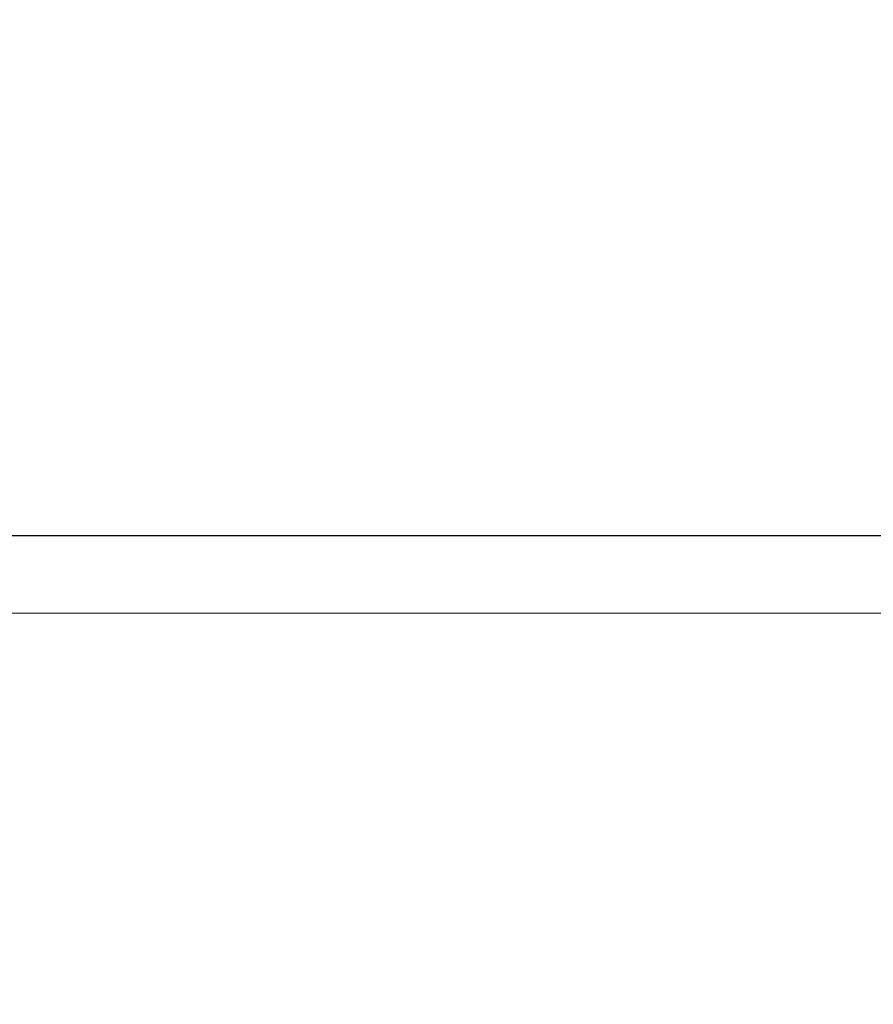
# Model space of a CAD drawing. Units: inches. Extents: x -1198 to -69, y -512 to 437.
# Tile 10 of 50: x -956.359 to -950.733, y 182.142 to 188.628. Entities that reach past the tile are written whole.
import ezdxf

# ---------------------------------------------------------------- set-up
doc = ezdxf.new("R2010")
doc.units = ezdxf.units.IN
doc.header["$MEASUREMENT"] = 0
for name, color, linetype, lineweight in [('0_Pen_No__7', 7, 'Continuous', 18), ('A-ANNO-DIMS', 2, 'Continuous', 18), ('A-EQPM', 60, 'Continuous', 18), ('A-FLOR-CASE', 7, 'Continuous', 25)]:
    doc.layers.add(name, color=color, linetype=linetype, lineweight=lineweight)
doc.styles.get("Standard").update_dxf_attribs({"font": 'arial.ttf'})
doc.dimstyles.get("Standard").update_dxf_attribs({"dimtxt": 6, "dimasz": 6, "dimexe": 0.18, "dimexo": 0.0625, "dimgap": 0.09, "dimtad": 0, "dimtih": 1, "dimtoh": 1, "dimdec": 0, "dimzin": 0, "dimdsep": 46, "dimlunit": 4, "dimtxsty": 'Standard', "dimblk": 'OBLIQUE', "dimcen": 0.09, "dimadec": 0, "dimazin": 0, "dimtfac": 1, "dimtdec": 0, "dimtofl": 0, "dimtmove": 0, "dimatfit": 3, "dimfxl": 1, "dimtolj": 1, "dimtzin": 0, "dimarcsym": 0})

# ---------------------------------------------------------------- blocks, each defined once
blk = doc.blocks.new('new block')
at = {"layer": '0_Pen_No__7'}
blk.add_lwpolyline([(-354.49, 596.91), (481.18, 596.91, -0.414214), (485.68, 592.4), (485.68, 99.11), (486.24, 99.11), (486.24, 95.73), (485.68, 95.73), (485.68, 4.5, -0.414214), (481.18, 0), (-354.49, 0, -0.414214), (-359, 4.5), (-359, 95.73), (-359.56, 95.73), (-359.56, 99.11), (-359, 99.11), (-359, 592.4, -0.414214)], format="xyb", close=True, dxfattribs=at)
blk.add_lwpolyline([(-333.7, 12.95), (460.3, 12.95), (460.3, 570.44), (-333.7, 570.44)], close=True, dxfattribs=at)
blk = doc.blocks.new('COUNTER-L')
at = {"ltscale": 10}
blk.add_line((49.3491, 23.9997), (0.0001, 23.9997), dxfattribs=at)
blk = doc.blocks.new('_Oblique')
at = {"color": 0, "linetype": 'ByBlock', "lineweight": -2}
blk.add_line((-0.5, -0.5), (0.5, 0.5), dxfattribs=at)
blk = doc.blocks.new('*D50')
at = {"layer": 'A-ANNO-DIMS', "color": 0, "lineweight": -2, "ltscale": 10, "transparency": 16777216}
for p, q in [((-978.4621, 185.2902), (-978.4621, 190.4026)), ((-945.1627, 185.2902), (-945.1627, 190.4026)), ((-978.4621, 190.2226), (-984.4621, 190.2226)), ((-945.1627, 190.2226), (-978.4621, 190.2226))]:
    blk.add_line(p, q, dxfattribs=at)
at = {"layer": 'DEFPOINTS', "color": 0, "ltscale": 10, "transparency": 16777216}
for p in [(-978.4621, 190.2226), (-978.4621, 185.2277), (-945.1627, 185.2277)]:
    blk.add_point(p, dxfattribs=at)
at = {"layer": 'A-ANNO-DIMS', "color": 0, "lineweight": -2, "ltscale": 10, "transparency": 16777216, "xscale": 6, "yscale": 6, "zscale": 6, "rotation": 180}
blk.add_blockref('_Oblique', (-978.4621, 190.2226), dxfattribs=at)
at = {"layer": 'A-ANNO-DIMS', "color": 0, "lineweight": -2, "ltscale": 10, "transparency": 16777216, "xscale": 6, "yscale": 6, "zscale": 6}
blk.add_blockref('_Oblique', (-945.1627, 190.2226), dxfattribs=at)
at = {"layer": 'A-ANNO-DIMS', "color": 0, "ltscale": 10, "transparency": 16777216, "insert": (-1009.2397, 190.2226), "char_height": 6, "attachment_point": 5}
blk.add_mtext('\\A1;HOB 33 TYP.', dxfattribs=at)

msp = doc.modelspace()

# ---------------------------------------------------------------- block references
at = {"layer": 'A-EQPM', "xscale": 0.0393700787401575, "yscale": 0.0393700787401575, "zscale": 0.0393700787401575, "rotation": 180}
msp.add_blockref('new block', (-959.3186, 185.2277), dxfattribs=at)
at = {"layer": 'A-FLOR-CASE'}
msp.add_blockref('COUNTER-L', (-988.751, 161.228), dxfattribs=at)

# ---------------------------------------------------------------- dimensions: what is measured, and where the dimension line sits
at = {"layer": 'A-ANNO-DIMS', "ltscale": 10}
dim = msp.add_linear_dim(base=(-978.4621, 190.2226), p1=(-945.1627, 185.2277), p2=(-978.4621, 185.2277), angle=180, text='HOB <> TYP.', dimstyle='Standard', override={"dimdec": 0, "dimlfac": 1, "dimrnd": 0, "dimzin": 0, "dimdsep": 46, "dimlunit": 2}, dxfattribs=at)
dim.commit()
dim.dimension.update_dxf_attribs({"geometry": '*D50', "text_midpoint": (-1009.2397, 190.2226)})

doc.saveas('drawing.dxf')
